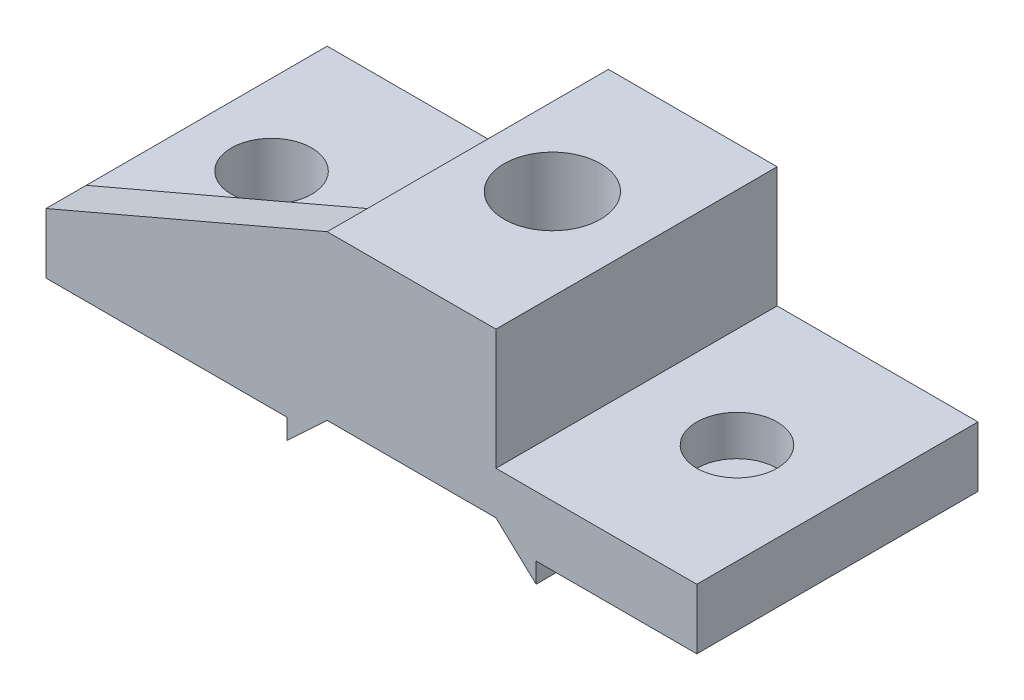
ISO-10303-21;
HEADER;
FILE_DESCRIPTION(('STEP AP214'),'2;1');
FILE_NAME('part.step','',(''),(''),'','','');
FILE_SCHEMA(('AUTOMOTIVE_DESIGN { 1 0 10303 214 1 1 1 1 }'));
ENDSEC;
DATA;
#1=APPLICATION_CONTEXT('core data for automotive mechanical design processes');
#2=APPLICATION_PROTOCOL_DEFINITION('international standard','automotive_design',2000,#1);
#3=PRODUCT_CONTEXT('',#1,'mechanical');
#4=PRODUCT('Part','Part','',(#3));
#5=PRODUCT_RELATED_PRODUCT_CATEGORY('part','',(#4));
#6=PRODUCT_DEFINITION_FORMATION('','',#4);
#7=PRODUCT_DEFINITION_CONTEXT('part definition',#1,'design');
#8=PRODUCT_DEFINITION('design','',#6,#7);
#9=PRODUCT_DEFINITION_SHAPE('','',#8);
#10=(LENGTH_UNIT() NAMED_UNIT(*) SI_UNIT(.MILLI.,.METRE.));
#11=(NAMED_UNIT(*) PLANE_ANGLE_UNIT() SI_UNIT($,.RADIAN.));
#12=(NAMED_UNIT(*) SI_UNIT($,.STERADIAN.) SOLID_ANGLE_UNIT());
#13=UNCERTAINTY_MEASURE_WITH_UNIT(LENGTH_MEASURE(1.E-05),#10,'distance_accuracy_value','');
#14=(GEOMETRIC_REPRESENTATION_CONTEXT(3) GLOBAL_UNCERTAINTY_ASSIGNED_CONTEXT((#13)) GLOBAL_UNIT_ASSIGNED_CONTEXT((#10,
#11,#12)) REPRESENTATION_CONTEXT('',''));
#15=CARTESIAN_POINT('',(0.,0.,0.));
#16=DIRECTION('',(0.,0.,1.));
#17=DIRECTION('',(1.,0.,0.));
#18=AXIS2_PLACEMENT_3D('',#15,#16,#17);
#19=CARTESIAN_POINT('',(70.,0.,70.));
#20=DIRECTION('',(0.,1.,0.));
#21=DIRECTION('',(0.,0.,1.));
#22=AXIS2_PLACEMENT_3D('',#19,#20,#21);
#23=PLANE('',#22);
#24=CARTESIAN_POINT('',(30.,0.,33.8565672520872));
#25=DIRECTION('',(0.,1.,0.));
#26=DIRECTION('',(0.,0.,1.));
#27=AXIS2_PLACEMENT_3D('',#24,#25,#26);
#28=CIRCLE('',#27,10.);
#29=CARTESIAN_POINT('',(30.,0.,43.8565672520872));
#30=VERTEX_POINT('',#29);
#31=EDGE_CURVE('E177',#30,#30,#28,.T.);
#32=ORIENTED_EDGE('',*,*,#31,.T.);
#33=EDGE_LOOP('',(#32));
#34=FACE_BOUND('',#33,.T.);
#35=DIRECTION('',(1.,0.,0.));
#36=VECTOR('',#35,1.);
#37=CARTESIAN_POINT('',(70.,0.,0.));
#38=LINE('',#37,#36);
#39=CARTESIAN_POINT('',(9.99999999999999,0.,0.));
#40=VERTEX_POINT('',#39);
#41=CARTESIAN_POINT('',(70.,0.,0.));
#42=VERTEX_POINT('',#41);
#43=EDGE_CURVE('E174',#40,#42,#38,.T.);
#44=ORIENTED_EDGE('',*,*,#43,.T.);
#45=DIRECTION('',(0.,0.,-1.));
#46=VECTOR('',#45,1.);
#47=CARTESIAN_POINT('',(70.,0.,70.));
#48=LINE('',#47,#46);
#49=CARTESIAN_POINT('',(70.,0.,70.));
#50=VERTEX_POINT('',#49);
#51=EDGE_CURVE('E11',#50,#42,#48,.T.);
#52=ORIENTED_EDGE('',*,*,#51,.F.);
#53=DIRECTION('',(1.,0.,0.));
#54=VECTOR('',#53,1.);
#55=CARTESIAN_POINT('',(70.,0.,70.));
#56=LINE('',#55,#54);
#57=CARTESIAN_POINT('',(9.99999999999999,0.,70.));
#58=VERTEX_POINT('',#57);
#59=EDGE_CURVE('E203',#58,#50,#56,.T.);
#60=ORIENTED_EDGE('',*,*,#59,.F.);
#61=DIRECTION('',(0.,0.,-1.));
#62=VECTOR('',#61,1.);
#63=CARTESIAN_POINT('',(9.99999999999999,0.,70.));
#64=LINE('',#63,#62);
#65=EDGE_CURVE('E171',#58,#40,#64,.T.);
#66=ORIENTED_EDGE('',*,*,#65,.T.);
#67=EDGE_LOOP('',(#44,#52,#60,#66));
#68=FACE_BOUND('',#67,.T.);
#69=ADVANCED_FACE('F39',(#34,#68),#23,.F.);
#70=CARTESIAN_POINT('',(70.,0.,70.));
#71=DIRECTION('',(1.,0.,0.));
#72=DIRECTION('',(0.,0.,-1.));
#73=AXIS2_PLACEMENT_3D('',#70,#71,#72);
#74=PLANE('',#73);
#75=DIRECTION('',(0.,-1.,0.));
#76=VECTOR('',#75,1.);
#77=CARTESIAN_POINT('',(70.,0.,0.));
#78=LINE('',#77,#76);
#79=CARTESIAN_POINT('',(70.,-5.,0.));
#80=VERTEX_POINT('',#79);
#81=EDGE_CURVE('E178',#42,#80,#78,.T.);
#82=ORIENTED_EDGE('',*,*,#81,.T.);
#83=DIRECTION('',(0.,0.,-1.));
#84=VECTOR('',#83,1.);
#85=CARTESIAN_POINT('',(70.,-5.,70.));
#86=LINE('',#85,#84);
#87=CARTESIAN_POINT('',(70.,-5.,70.));
#88=VERTEX_POINT('',#87);
#89=EDGE_CURVE('E50',#88,#80,#86,.T.);
#90=ORIENTED_EDGE('',*,*,#89,.F.);
#91=DIRECTION('',(0.,-1.,0.));
#92=VECTOR('',#91,1.);
#93=CARTESIAN_POINT('',(70.,0.,70.));
#94=LINE('',#93,#92);
#95=EDGE_CURVE('E114',#50,#88,#94,.T.);
#96=ORIENTED_EDGE('',*,*,#95,.F.);
#97=ORIENTED_EDGE('',*,*,#51,.T.);
#98=EDGE_LOOP('',(#82,#90,#96,#97));
#99=FACE_BOUND('',#98,.T.);
#100=ADVANCED_FACE('F309',(#99),#74,.F.);
#101=CARTESIAN_POINT('',(70.,-5.,70.));
#102=DIRECTION('',(-0.681759867063012,0.731576027260478,0.));
#103=DIRECTION('',(-0.731576027260478,-0.681759867063012,0.));
#104=AXIS2_PLACEMENT_3D('',#101,#102,#103);
#105=PLANE('',#104);
#106=DIRECTION('',(0.731576027260478,0.681759867063012,0.));
#107=VECTOR('',#106,1.);
#108=CARTESIAN_POINT('',(70.,-5.,0.));
#109=LINE('',#108,#107);
#110=CARTESIAN_POINT('',(80.,4.31905696276008,0.));
#111=VERTEX_POINT('',#110);
#112=EDGE_CURVE('E181',#80,#111,#109,.T.);
#113=ORIENTED_EDGE('',*,*,#112,.T.);
#114=DIRECTION('',(0.,0.,-1.));
#115=VECTOR('',#114,1.);
#116=CARTESIAN_POINT('',(80.,4.31905696276008,70.));
#117=LINE('',#116,#115);
#118=CARTESIAN_POINT('',(80.,4.31905696276008,70.));
#119=VERTEX_POINT('',#118);
#120=EDGE_CURVE('E226',#119,#111,#117,.T.);
#121=ORIENTED_EDGE('',*,*,#120,.F.);
#122=DIRECTION('',(0.731576027260478,0.681759867063012,0.));
#123=VECTOR('',#122,1.);
#124=CARTESIAN_POINT('',(70.,-5.,70.));
#125=LINE('',#124,#123);
#126=EDGE_CURVE('E236',#88,#119,#125,.T.);
#127=ORIENTED_EDGE('',*,*,#126,.F.);
#128=ORIENTED_EDGE('',*,*,#89,.T.);
#129=EDGE_LOOP('',(#113,#121,#127,#128));
#130=FACE_BOUND('',#129,.T.);
#131=ADVANCED_FACE('F234',(#130),#105,.F.);
#132=CARTESIAN_POINT('',(80.,4.31905696276008,70.));
#133=DIRECTION('',(0.,1.,0.));
#134=DIRECTION('',(0.,0.,1.));
#135=AXIS2_PLACEMENT_3D('',#132,#133,#134);
#136=PLANE('',#135);
#137=DIRECTION('',(1.,0.,0.));
#138=VECTOR('',#137,1.);
#139=CARTESIAN_POINT('',(80.,4.31905696276008,0.));
#140=LINE('',#139,#138);
#141=CARTESIAN_POINT('',(122.,4.31905696276008,0.));
#142=VERTEX_POINT('',#141);
#143=EDGE_CURVE('E182',#111,#142,#140,.T.);
#144=ORIENTED_EDGE('',*,*,#143,.T.);
#145=DIRECTION('',(0.,0.,-1.));
#146=VECTOR('',#145,1.);
#147=CARTESIAN_POINT('',(122.,4.31905696276008,70.));
#148=LINE('',#147,#146);
#149=CARTESIAN_POINT('',(122.,4.31905696276008,70.));
#150=VERTEX_POINT('',#149);
#151=EDGE_CURVE('E225',#150,#142,#148,.T.);
#152=ORIENTED_EDGE('',*,*,#151,.F.);
#153=DIRECTION('',(1.,0.,0.));
#154=VECTOR('',#153,1.);
#155=CARTESIAN_POINT('',(80.,4.31905696276008,70.));
#156=LINE('',#155,#154);
#157=EDGE_CURVE('E251',#119,#150,#156,.T.);
#158=ORIENTED_EDGE('',*,*,#157,.F.);
#159=ORIENTED_EDGE('',*,*,#120,.T.);
#160=EDGE_LOOP('',(#144,#152,#158,#159));
#161=FACE_BOUND('',#160,.T.);
#162=ADVANCED_FACE('F244',(#161),#136,.F.);
#163=CARTESIAN_POINT('',(122.,4.31905696276008,70.));
#164=DIRECTION('',(0.681759867063012,0.731576027260478,0.));
#165=DIRECTION('',(-0.731576027260478,0.681759867063012,0.));
#166=AXIS2_PLACEMENT_3D('',#163,#164,#165);
#167=PLANE('',#166);
#168=DIRECTION('',(0.731576027260478,-0.681759867063012,0.));
#169=VECTOR('',#168,1.);
#170=CARTESIAN_POINT('',(122.,4.31905696276008,0.));
#171=LINE('',#170,#169);
#172=CARTESIAN_POINT('',(132.,-5.,0.));
#173=VERTEX_POINT('',#172);
#174=EDGE_CURVE('E184',#142,#173,#171,.T.);
#175=ORIENTED_EDGE('',*,*,#174,.T.);
#176=DIRECTION('',(0.,0.,-1.));
#177=VECTOR('',#176,1.);
#178=CARTESIAN_POINT('',(132.,-5.,70.));
#179=LINE('',#178,#177);
#180=CARTESIAN_POINT('',(132.,-5.,70.));
#181=VERTEX_POINT('',#180);
#182=EDGE_CURVE('E222',#181,#173,#179,.T.);
#183=ORIENTED_EDGE('',*,*,#182,.F.);
#184=DIRECTION('',(0.731576027260478,-0.681759867063012,0.));
#185=VECTOR('',#184,1.);
#186=CARTESIAN_POINT('',(122.,4.31905696276008,70.));
#187=LINE('',#186,#185);
#188=EDGE_CURVE('E252',#150,#181,#187,.T.);
#189=ORIENTED_EDGE('',*,*,#188,.F.);
#190=ORIENTED_EDGE('',*,*,#151,.T.);
#191=EDGE_LOOP('',(#175,#183,#189,#190));
#192=FACE_BOUND('',#191,.T.);
#193=ADVANCED_FACE('F248',(#192),#167,.F.);
#194=CARTESIAN_POINT('',(132.,-5.,70.));
#195=DIRECTION('',(-1.,0.,0.));
#196=DIRECTION('',(0.,0.,1.));
#197=AXIS2_PLACEMENT_3D('',#194,#195,#196);
#198=PLANE('',#197);
#199=DIRECTION('',(0.,1.,0.));
#200=VECTOR('',#199,1.);
#201=CARTESIAN_POINT('',(132.,-5.,0.));
#202=LINE('',#201,#200);
#203=CARTESIAN_POINT('',(132.,0.,0.));
#204=VERTEX_POINT('',#203);
#205=EDGE_CURVE('E190',#173,#204,#202,.T.);
#206=ORIENTED_EDGE('',*,*,#205,.T.);
#207=DIRECTION('',(0.,0.,-1.));
#208=VECTOR('',#207,1.);
#209=CARTESIAN_POINT('',(132.,0.,70.));
#210=LINE('',#209,#208);
#211=CARTESIAN_POINT('',(132.,0.,70.));
#212=VERTEX_POINT('',#211);
#213=EDGE_CURVE('E216',#212,#204,#210,.T.);
#214=ORIENTED_EDGE('',*,*,#213,.F.);
#215=DIRECTION('',(0.,1.,0.));
#216=VECTOR('',#215,1.);
#217=CARTESIAN_POINT('',(132.,-5.,70.));
#218=LINE('',#217,#216);
#219=EDGE_CURVE('E254',#181,#212,#218,.T.);
#220=ORIENTED_EDGE('',*,*,#219,.F.);
#221=ORIENTED_EDGE('',*,*,#182,.T.);
#222=EDGE_LOOP('',(#206,#214,#220,#221));
#223=FACE_BOUND('',#222,.T.);
#224=ADVANCED_FACE('F325',(#223),#198,.F.);
#225=CARTESIAN_POINT('',(132.,0.,70.));
#226=DIRECTION('',(0.,1.,0.));
#227=DIRECTION('',(0.,0.,1.));
#228=AXIS2_PLACEMENT_3D('',#225,#226,#227);
#229=PLANE('',#228);
#230=DIRECTION('',(1.,0.,0.));
#231=VECTOR('',#230,1.);
#232=CARTESIAN_POINT('',(132.,0.,0.));
#233=LINE('',#232,#231);
#234=CARTESIAN_POINT('',(172.,0.,0.));
#235=VERTEX_POINT('',#234);
#236=EDGE_CURVE('E186',#204,#235,#233,.T.);
#237=ORIENTED_EDGE('',*,*,#236,.T.);
#238=DIRECTION('',(0.,0.,-1.));
#239=VECTOR('',#238,1.);
#240=CARTESIAN_POINT('',(172.,0.,70.));
#241=LINE('',#240,#239);
#242=CARTESIAN_POINT('',(172.,0.,70.));
#243=VERTEX_POINT('',#242);
#244=EDGE_CURVE('E217',#243,#235,#241,.T.);
#245=ORIENTED_EDGE('',*,*,#244,.F.);
#246=DIRECTION('',(1.,0.,0.));
#247=VECTOR('',#246,1.);
#248=CARTESIAN_POINT('',(132.,0.,70.));
#249=LINE('',#248,#247);
#250=EDGE_CURVE('E259',#212,#243,#249,.T.);
#251=ORIENTED_EDGE('',*,*,#250,.F.);
#252=ORIENTED_EDGE('',*,*,#213,.T.);
#253=EDGE_LOOP('',(#237,#245,#251,#252));
#254=FACE_BOUND('',#253,.T.);
#255=ADVANCED_FACE('F327',(#254),#229,.F.);
#256=CARTESIAN_POINT('',(172.,0.,70.));
#257=DIRECTION('',(-1.,0.,0.));
#258=DIRECTION('',(0.,0.,1.));
#259=AXIS2_PLACEMENT_3D('',#256,#257,#258);
#260=PLANE('',#259);
#261=DIRECTION('',(0.,1.,0.));
#262=VECTOR('',#261,1.);
#263=CARTESIAN_POINT('',(172.,0.,0.));
#264=LINE('',#263,#262);
#265=CARTESIAN_POINT('',(172.,15.,0.));
#266=VERTEX_POINT('',#265);
#267=EDGE_CURVE('E194',#235,#266,#264,.T.);
#268=ORIENTED_EDGE('',*,*,#267,.T.);
#269=DIRECTION('',(0.,0.,-1.));
#270=VECTOR('',#269,1.);
#271=CARTESIAN_POINT('',(172.,15.,70.));
#272=LINE('',#271,#270);
#273=CARTESIAN_POINT('',(172.,15.,70.));
#274=VERTEX_POINT('',#273);
#275=EDGE_CURVE('E215',#274,#266,#272,.T.);
#276=ORIENTED_EDGE('',*,*,#275,.F.);
#277=DIRECTION('',(0.,1.,0.));
#278=VECTOR('',#277,1.);
#279=CARTESIAN_POINT('',(172.,0.,70.));
#280=LINE('',#279,#278);
#281=EDGE_CURVE('E265',#243,#274,#280,.T.);
#282=ORIENTED_EDGE('',*,*,#281,.F.);
#283=ORIENTED_EDGE('',*,*,#244,.T.);
#284=EDGE_LOOP('',(#268,#276,#282,#283));
#285=FACE_BOUND('',#284,.T.);
#286=ADVANCED_FACE('F269',(#285),#260,.F.);
#287=CARTESIAN_POINT('',(172.,15.,70.));
#288=DIRECTION('',(0.,-1.,0.));
#289=DIRECTION('',(0.,0.,-1.));
#290=AXIS2_PLACEMENT_3D('',#287,#288,#289);
#291=PLANE('',#290);
#292=CARTESIAN_POINT('',(147.,15.,35.));
#293=DIRECTION('',(0.,1.,0.));
#294=DIRECTION('',(0.,0.,1.));
#295=AXIS2_PLACEMENT_3D('',#292,#293,#294);
#296=CIRCLE('',#295,10.);
#297=CARTESIAN_POINT('',(147.,15.,45.));
#298=VERTEX_POINT('',#297);
#299=EDGE_CURVE('E381',#298,#298,#296,.T.);
#300=ORIENTED_EDGE('',*,*,#299,.F.);
#301=EDGE_LOOP('',(#300));
#302=FACE_BOUND('',#301,.T.);
#303=DIRECTION('',(-1.,0.,0.));
#304=VECTOR('',#303,1.);
#305=CARTESIAN_POINT('',(172.,15.,0.));
#306=LINE('',#305,#304);
#307=CARTESIAN_POINT('',(122.,15.,0.));
#308=VERTEX_POINT('',#307);
#309=EDGE_CURVE('E195',#266,#308,#306,.T.);
#310=ORIENTED_EDGE('',*,*,#309,.T.);
#311=DIRECTION('',(0.,0.,-1.));
#312=VECTOR('',#311,1.);
#313=CARTESIAN_POINT('',(122.,15.,70.));
#314=LINE('',#313,#312);
#315=CARTESIAN_POINT('',(122.,15.,70.));
#316=VERTEX_POINT('',#315);
#317=EDGE_CURVE('E165',#316,#308,#314,.T.);
#318=ORIENTED_EDGE('',*,*,#317,.F.);
#319=DIRECTION('',(-1.,0.,0.));
#320=VECTOR('',#319,1.);
#321=CARTESIAN_POINT('',(172.,15.,70.));
#322=LINE('',#321,#320);
#323=EDGE_CURVE('E152',#274,#316,#322,.T.);
#324=ORIENTED_EDGE('',*,*,#323,.F.);
#325=ORIENTED_EDGE('',*,*,#275,.T.);
#326=EDGE_LOOP('',(#310,#318,#324,#325));
#327=FACE_BOUND('',#326,.T.);
#328=ADVANCED_FACE('F275',(#302,#327),#291,.F.);
#329=CARTESIAN_POINT('',(122.,15.,70.));
#330=DIRECTION('',(-1.,0.,0.));
#331=DIRECTION('',(0.,0.,1.));
#332=AXIS2_PLACEMENT_3D('',#329,#330,#331);
#333=PLANE('',#332);
#334=DIRECTION('',(0.,1.,0.));
#335=VECTOR('',#334,1.);
#336=CARTESIAN_POINT('',(122.,15.,0.));
#337=LINE('',#336,#335);
#338=CARTESIAN_POINT('',(122.,45.,0.));
#339=VERTEX_POINT('',#338);
#340=EDGE_CURVE('E160',#308,#339,#337,.T.);
#341=ORIENTED_EDGE('',*,*,#340,.T.);
#342=DIRECTION('',(0.,0.,-1.));
#343=VECTOR('',#342,1.);
#344=CARTESIAN_POINT('',(122.,45.,70.));
#345=LINE('',#344,#343);
#346=CARTESIAN_POINT('',(122.,45.,70.));
#347=VERTEX_POINT('',#346);
#348=EDGE_CURVE('E157',#347,#339,#345,.T.);
#349=ORIENTED_EDGE('',*,*,#348,.F.);
#350=DIRECTION('',(0.,1.,0.));
#351=VECTOR('',#350,1.);
#352=CARTESIAN_POINT('',(122.,15.,70.));
#353=LINE('',#352,#351);
#354=EDGE_CURVE('E144',#316,#347,#353,.T.);
#355=ORIENTED_EDGE('',*,*,#354,.F.);
#356=ORIENTED_EDGE('',*,*,#317,.T.);
#357=EDGE_LOOP('',(#341,#349,#355,#356));
#358=FACE_BOUND('',#357,.T.);
#359=ADVANCED_FACE('F159',(#358),#333,.F.);
#360=CARTESIAN_POINT('',(122.,45.,70.));
#361=DIRECTION('',(0.,-1.,0.));
#362=DIRECTION('',(1.,0.,0.));
#363=AXIS2_PLACEMENT_3D('',#360,#361,#362);
#364=PLANE('',#363);
#365=CARTESIAN_POINT('',(99.3471690358092,45.,33.2963544432801));
#366=DIRECTION('',(0.,1.,0.));
#367=DIRECTION('',(-1.,0.,0.));
#368=AXIS2_PLACEMENT_3D('',#365,#366,#367);
#369=CIRCLE('',#368,12.);
#370=CARTESIAN_POINT('',(87.3471690358092,45.,33.2963544432801));
#371=VERTEX_POINT('',#370);
#372=EDGE_CURVE('E286',#371,#371,#369,.T.);
#373=ORIENTED_EDGE('',*,*,#372,.F.);
#374=EDGE_LOOP('',(#373));
#375=FACE_BOUND('',#374,.T.);
#376=DIRECTION('',(-1.,0.,0.));
#377=VECTOR('',#376,1.);
#378=CARTESIAN_POINT('',(122.,45.,0.));
#379=LINE('',#378,#377);
#380=CARTESIAN_POINT('',(80.,45.,0.));
#381=VERTEX_POINT('',#380);
#382=EDGE_CURVE('E197',#339,#381,#379,.T.);
#383=ORIENTED_EDGE('',*,*,#382,.T.);
#384=DIRECTION('',(0.,0.,-1.));
#385=VECTOR('',#384,1.);
#386=CARTESIAN_POINT('',(80.,45.,70.));
#387=LINE('',#386,#385);
#388=CARTESIAN_POINT('',(80.,45.,60.));
#389=VERTEX_POINT('',#388);
#390=EDGE_CURVE('E208',#389,#381,#387,.T.);
#391=ORIENTED_EDGE('',*,*,#390,.F.);
#392=CARTESIAN_POINT('',(80.,45.,70.));
#393=VERTEX_POINT('',#392);
#394=EDGE_CURVE('E164',#393,#389,#387,.T.);
#395=ORIENTED_EDGE('',*,*,#394,.F.);
#396=DIRECTION('',(-1.,0.,0.));
#397=VECTOR('',#396,1.);
#398=CARTESIAN_POINT('',(122.,45.,70.));
#399=LINE('',#398,#397);
#400=EDGE_CURVE('E150',#347,#393,#399,.T.);
#401=ORIENTED_EDGE('',*,*,#400,.F.);
#402=ORIENTED_EDGE('',*,*,#348,.T.);
#403=EDGE_LOOP('',(#383,#391,#395,#401,#402));
#404=FACE_BOUND('',#403,.T.);
#405=ADVANCED_FACE('F170',(#375,#404),#364,.F.);
#406=CARTESIAN_POINT('',(80.,45.,70.));
#407=DIRECTION('',(1.,0.,0.));
#408=DIRECTION('',(0.,0.,-1.));
#409=AXIS2_PLACEMENT_3D('',#406,#407,#408);
#410=PLANE('',#409);
#411=DIRECTION('',(0.,0.,-1.));
#412=VECTOR('',#411,1.);
#413=CARTESIAN_POINT('',(80.,15.,70.));
#414=LINE('',#413,#412);
#415=CARTESIAN_POINT('',(80.,15.,60.));
#416=VERTEX_POINT('',#415);
#417=CARTESIAN_POINT('',(80.,15.,0.));
#418=VERTEX_POINT('',#417);
#419=EDGE_CURVE('E206',#416,#418,#414,.T.);
#420=ORIENTED_EDGE('',*,*,#419,.F.);
#421=DIRECTION('',(0.,1.,0.));
#422=VECTOR('',#421,1.);
#423=CARTESIAN_POINT('',(80.,15.,60.));
#424=LINE('',#423,#422);
#425=EDGE_CURVE('E282',#416,#389,#424,.T.);
#426=ORIENTED_EDGE('',*,*,#425,.T.);
#427=ORIENTED_EDGE('',*,*,#390,.T.);
#428=DIRECTION('',(0.,-1.,0.));
#429=VECTOR('',#428,1.);
#430=CARTESIAN_POINT('',(80.,45.,0.));
#431=LINE('',#430,#429);
#432=EDGE_CURVE('E199',#381,#418,#431,.T.);
#433=ORIENTED_EDGE('',*,*,#432,.T.);
#434=EDGE_LOOP('',(#420,#426,#427,#433));
#435=FACE_BOUND('',#434,.T.);
#436=ADVANCED_FACE('F278',(#435),#410,.F.);
#437=CARTESIAN_POINT('',(9.99999999999999,15.,70.));
#438=DIRECTION('',(0.,-1.,0.));
#439=DIRECTION('',(0.,0.,-1.));
#440=AXIS2_PLACEMENT_3D('',#437,#438,#439);
#441=PLANE('',#440);
#442=CARTESIAN_POINT('',(30.,15.,33.8565672520872));
#443=DIRECTION('',(0.,1.,0.));
#444=DIRECTION('',(0.,0.,1.));
#445=AXIS2_PLACEMENT_3D('',#442,#443,#444);
#446=CIRCLE('',#445,10.);
#447=CARTESIAN_POINT('',(30.,15.,43.8565672520872));
#448=VERTEX_POINT('',#447);
#449=EDGE_CURVE('E297',#448,#448,#446,.T.);
#450=ORIENTED_EDGE('',*,*,#449,.F.);
#451=EDGE_LOOP('',(#450));
#452=FACE_BOUND('',#451,.T.);
#453=DIRECTION('',(0.,0.,-1.));
#454=VECTOR('',#453,1.);
#455=CARTESIAN_POINT('',(9.99999999999999,15.,70.));
#456=LINE('',#455,#454);
#457=CARTESIAN_POINT('',(9.99999999999999,15.,60.));
#458=VERTEX_POINT('',#457);
#459=CARTESIAN_POINT('',(9.99999999999999,15.,0.));
#460=VERTEX_POINT('',#459);
#461=EDGE_CURVE('E101',#458,#460,#456,.T.);
#462=ORIENTED_EDGE('',*,*,#461,.F.);
#463=DIRECTION('',(1.,0.,0.));
#464=VECTOR('',#463,1.);
#465=CARTESIAN_POINT('',(9.99999999999999,15.,60.));
#466=LINE('',#465,#464);
#467=EDGE_CURVE('E287',#458,#416,#466,.T.);
#468=ORIENTED_EDGE('',*,*,#467,.T.);
#469=ORIENTED_EDGE('',*,*,#419,.T.);
#470=DIRECTION('',(-1.,0.,0.));
#471=VECTOR('',#470,1.);
#472=CARTESIAN_POINT('',(9.99999999999999,15.,0.));
#473=LINE('',#472,#471);
#474=EDGE_CURVE('E201',#418,#460,#473,.T.);
#475=ORIENTED_EDGE('',*,*,#474,.T.);
#476=EDGE_LOOP('',(#462,#468,#469,#475));
#477=FACE_BOUND('',#476,.T.);
#478=ADVANCED_FACE('F345',(#452,#477),#441,.F.);
#479=CARTESIAN_POINT('',(9.99999999999999,0.,70.));
#480=DIRECTION('',(1.,0.,0.));
#481=DIRECTION('',(0.,0.,-1.));
#482=AXIS2_PLACEMENT_3D('',#479,#480,#481);
#483=PLANE('',#482);
#484=DIRECTION('',(0.,-1.,0.));
#485=VECTOR('',#484,1.);
#486=CARTESIAN_POINT('',(9.99999999999999,0.,0.));
#487=LINE('',#486,#485);
#488=EDGE_CURVE('E110',#460,#40,#487,.T.);
#489=ORIENTED_EDGE('',*,*,#488,.T.);
#490=ORIENTED_EDGE('',*,*,#65,.F.);
#491=DIRECTION('',(0.,-1.,0.));
#492=VECTOR('',#491,1.);
#493=CARTESIAN_POINT('',(9.99999999999999,0.,70.));
#494=LINE('',#493,#492);
#495=CARTESIAN_POINT('',(9.99999999999999,15.,70.));
#496=VERTEX_POINT('',#495);
#497=EDGE_CURVE('E54',#496,#58,#494,.T.);
#498=ORIENTED_EDGE('',*,*,#497,.F.);
#499=EDGE_CURVE('E207',#496,#458,#456,.T.);
#500=ORIENTED_EDGE('',*,*,#499,.T.);
#501=ORIENTED_EDGE('',*,*,#461,.T.);
#502=EDGE_LOOP('',(#489,#490,#498,#500,#501));
#503=FACE_BOUND('',#502,.T.);
#504=ADVANCED_FACE('F347',(#503),#483,.F.);
#505=CARTESIAN_POINT('',(0.,0.,70.));
#506=DIRECTION('',(0.,0.,-1.));
#507=DIRECTION('',(-1.,0.,0.));
#508=AXIS2_PLACEMENT_3D('',#505,#506,#507);
#509=PLANE('',#508);
#510=ORIENTED_EDGE('',*,*,#59,.T.);
#511=ORIENTED_EDGE('',*,*,#95,.T.);
#512=ORIENTED_EDGE('',*,*,#126,.T.);
#513=ORIENTED_EDGE('',*,*,#157,.T.);
#514=ORIENTED_EDGE('',*,*,#188,.T.);
#515=ORIENTED_EDGE('',*,*,#219,.T.);
#516=ORIENTED_EDGE('',*,*,#250,.T.);
#517=ORIENTED_EDGE('',*,*,#281,.T.);
#518=ORIENTED_EDGE('',*,*,#323,.T.);
#519=ORIENTED_EDGE('',*,*,#354,.T.);
#520=ORIENTED_EDGE('',*,*,#400,.T.);
#521=DIRECTION('',(-0.919145030018058,-0.393919298579168,0.));
#522=VECTOR('',#521,1.);
#523=CARTESIAN_POINT('',(80.,45.,70.));
#524=LINE('',#523,#522);
#525=EDGE_CURVE('E298',#393,#496,#524,.T.);
#526=ORIENTED_EDGE('',*,*,#525,.T.);
#527=ORIENTED_EDGE('',*,*,#497,.T.);
#528=EDGE_LOOP('',(#510,#511,#512,#513,#514,#515,#516,#517,#518,#519,#520,#526,#527));
#529=FACE_BOUND('',#528,.T.);
#530=ADVANCED_FACE('F149',(#529),#509,.F.);
#531=CARTESIAN_POINT('',(0.,0.,0.));
#532=DIRECTION('',(0.,0.,-1.));
#533=DIRECTION('',(-1.,0.,0.));
#534=AXIS2_PLACEMENT_3D('',#531,#532,#533);
#535=PLANE('',#534);
#536=ORIENTED_EDGE('',*,*,#43,.F.);
#537=ORIENTED_EDGE('',*,*,#488,.F.);
#538=ORIENTED_EDGE('',*,*,#474,.F.);
#539=ORIENTED_EDGE('',*,*,#432,.F.);
#540=ORIENTED_EDGE('',*,*,#382,.F.);
#541=ORIENTED_EDGE('',*,*,#340,.F.);
#542=ORIENTED_EDGE('',*,*,#309,.F.);
#543=ORIENTED_EDGE('',*,*,#267,.F.);
#544=ORIENTED_EDGE('',*,*,#236,.F.);
#545=ORIENTED_EDGE('',*,*,#205,.F.);
#546=ORIENTED_EDGE('',*,*,#174,.F.);
#547=ORIENTED_EDGE('',*,*,#143,.F.);
#548=ORIENTED_EDGE('',*,*,#112,.F.);
#549=ORIENTED_EDGE('',*,*,#81,.F.);
#550=EDGE_LOOP('',(#536,#537,#538,#539,#540,#541,#542,#543,#544,#545,#546,#547,#548,#549));
#551=FACE_BOUND('',#550,.T.);
#552=ADVANCED_FACE('F239',(#551),#535,.T.);
#553=CARTESIAN_POINT('',(30.,-5.,33.8565672520872));
#554=DIRECTION('',(0.,1.,0.));
#555=DIRECTION('',(0.,0.,1.));
#556=AXIS2_PLACEMENT_3D('',#553,#554,#555);
#557=CYLINDRICAL_SURFACE('',#556,10.);
#558=ORIENTED_EDGE('',*,*,#449,.T.);
#559=EDGE_LOOP('',(#558));
#560=FACE_BOUND('',#559,.T.);
#561=ORIENTED_EDGE('',*,*,#31,.F.);
#562=EDGE_LOOP('',(#561));
#563=FACE_BOUND('',#562,.T.);
#564=ADVANCED_FACE('F352',(#560,#563),#557,.F.);
#565=CARTESIAN_POINT('',(99.3471690358092,25.,33.2963544432801));
#566=DIRECTION('',(0.,1.,0.));
#567=DIRECTION('',(-1.,0.,0.));
#568=AXIS2_PLACEMENT_3D('',#565,#566,#567);
#569=CYLINDRICAL_SURFACE('',#568,12.);
#570=CARTESIAN_POINT('',(99.3471690358092,25.,33.2963544432801));
#571=DIRECTION('',(0.,1.,0.));
#572=DIRECTION('',(-1.,0.,0.));
#573=AXIS2_PLACEMENT_3D('',#570,#571,#572);
#574=CIRCLE('',#573,12.);
#575=CARTESIAN_POINT('',(87.3471690358092,25.,33.2963544432801));
#576=VERTEX_POINT('',#575);
#577=EDGE_CURVE('E290',#576,#576,#574,.T.);
#578=ORIENTED_EDGE('',*,*,#577,.F.);
#579=EDGE_LOOP('',(#578));
#580=FACE_BOUND('',#579,.T.);
#581=ORIENTED_EDGE('',*,*,#372,.T.);
#582=EDGE_LOOP('',(#581));
#583=FACE_BOUND('',#582,.T.);
#584=ADVANCED_FACE('F357',(#580,#583),#569,.F.);
#585=CARTESIAN_POINT('',(99.3471690358092,25.,33.2963544432801));
#586=DIRECTION('',(0.,1.,0.));
#587=DIRECTION('',(-1.,0.,0.));
#588=AXIS2_PLACEMENT_3D('',#585,#586,#587);
#589=PLANE('',#588);
#590=ORIENTED_EDGE('',*,*,#577,.T.);
#591=EDGE_LOOP('',(#590));
#592=FACE_BOUND('',#591,.T.);
#593=ADVANCED_FACE('F363',(#592),#589,.T.);
#594=CARTESIAN_POINT('',(80.,45.,60.));
#595=DIRECTION('',(-0.393919298579168,0.919145030018058,0.));
#596=DIRECTION('',(-0.919145030018058,-0.393919298579168,0.));
#597=AXIS2_PLACEMENT_3D('',#594,#595,#596);
#598=PLANE('',#597);
#599=ORIENTED_EDGE('',*,*,#525,.F.);
#600=ORIENTED_EDGE('',*,*,#394,.T.);
#601=DIRECTION('',(-0.919145030018058,-0.393919298579168,0.));
#602=VECTOR('',#601,1.);
#603=CARTESIAN_POINT('',(80.,45.,60.));
#604=LINE('',#603,#602);
#605=EDGE_CURVE('E292',#389,#458,#604,.T.);
#606=ORIENTED_EDGE('',*,*,#605,.T.);
#607=ORIENTED_EDGE('',*,*,#499,.F.);
#608=EDGE_LOOP('',(#599,#600,#606,#607));
#609=FACE_BOUND('',#608,.T.);
#610=ADVANCED_FACE('F362',(#609),#598,.T.);
#611=CARTESIAN_POINT('',(0.,0.,60.));
#612=DIRECTION('',(0.,0.,-1.));
#613=DIRECTION('',(-1.,0.,0.));
#614=AXIS2_PLACEMENT_3D('',#611,#612,#613);
#615=PLANE('',#614);
#616=ORIENTED_EDGE('',*,*,#605,.F.);
#617=ORIENTED_EDGE('',*,*,#425,.F.);
#618=ORIENTED_EDGE('',*,*,#467,.F.);
#619=EDGE_LOOP('',(#616,#617,#618));
#620=FACE_BOUND('',#619,.T.);
#621=ADVANCED_FACE('F367',(#620),#615,.T.);
#622=CARTESIAN_POINT('',(147.,5.,35.));
#623=DIRECTION('',(0.,1.,0.));
#624=DIRECTION('',(0.,0.,1.));
#625=AXIS2_PLACEMENT_3D('',#622,#623,#624);
#626=CYLINDRICAL_SURFACE('',#625,10.);
#627=CARTESIAN_POINT('',(147.,5.,35.));
#628=DIRECTION('',(0.,1.,0.));
#629=DIRECTION('',(0.,0.,1.));
#630=AXIS2_PLACEMENT_3D('',#627,#628,#629);
#631=CIRCLE('',#630,10.);
#632=CARTESIAN_POINT('',(147.,5.,45.));
#633=VERTEX_POINT('',#632);
#634=EDGE_CURVE('E296',#633,#633,#631,.T.);
#635=ORIENTED_EDGE('',*,*,#634,.F.);
#636=EDGE_LOOP('',(#635));
#637=FACE_BOUND('',#636,.T.);
#638=ORIENTED_EDGE('',*,*,#299,.T.);
#639=EDGE_LOOP('',(#638));
#640=FACE_BOUND('',#639,.T.);
#641=ADVANCED_FACE('F373',(#637,#640),#626,.F.);
#642=CARTESIAN_POINT('',(147.,5.,35.));
#643=DIRECTION('',(0.,1.,0.));
#644=DIRECTION('',(0.,0.,1.));
#645=AXIS2_PLACEMENT_3D('',#642,#643,#644);
#646=PLANE('',#645);
#647=ORIENTED_EDGE('',*,*,#634,.T.);
#648=EDGE_LOOP('',(#647));
#649=FACE_BOUND('',#648,.T.);
#650=ADVANCED_FACE('F376',(#649),#646,.T.);
#651=CLOSED_SHELL('',(#69,#100,#131,#162,#193,#224,#255,#286,#328,#359,#405,#436,#478,#504,#530,
#552,#564,#584,#593,#610,#621,#641,#650));
#652=MANIFOLD_SOLID_BREP('B2',#651);
#653=ADVANCED_BREP_SHAPE_REPRESENTATION('',(#18,#652),#14);
#654=SHAPE_DEFINITION_REPRESENTATION(#9,#653);
ENDSEC;
END-ISO-10303-21;
